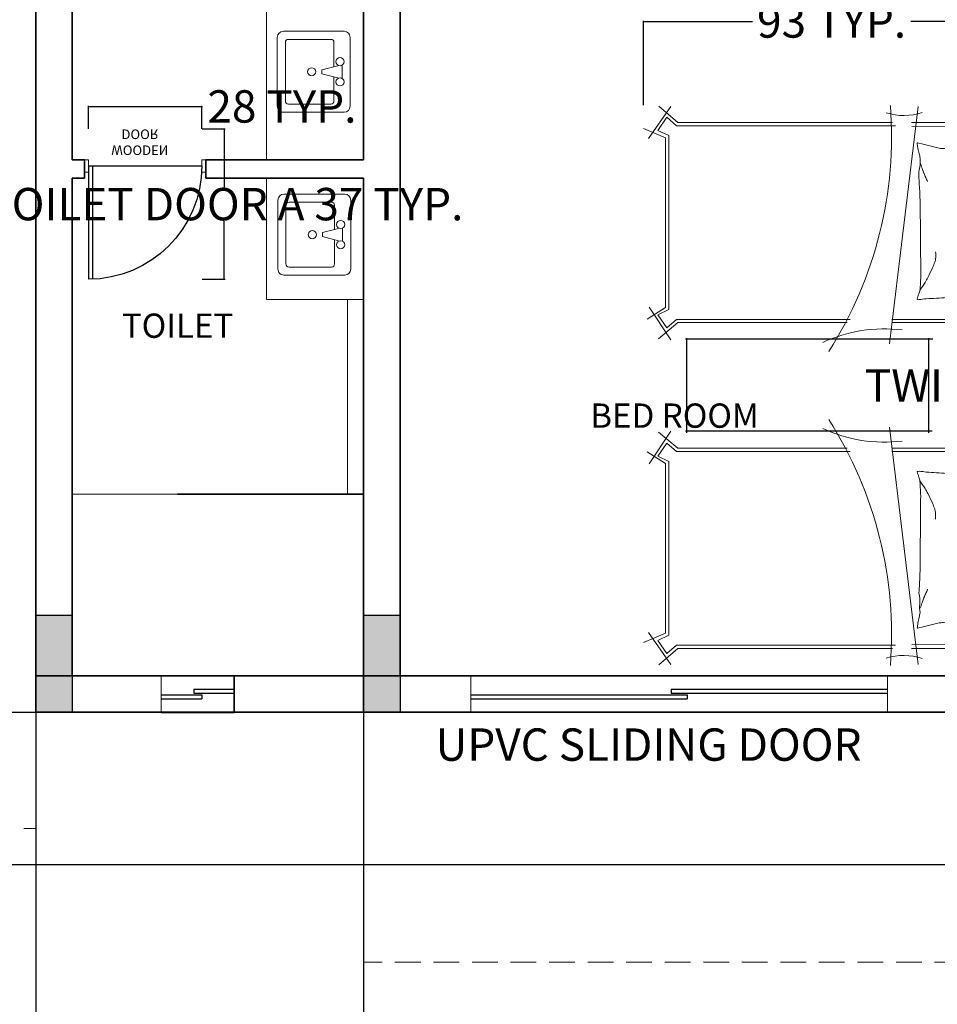
# Model space of a CAD drawing. Units: inches. Extents: x -48 to 50072, y 0 to 21068.
# Tile 51 of 75: x 212 to 439, y 417 to 660. Entities that reach past the tile are written whole.
import ezdxf

# ---------------------------------------------------------------- set-up
doc = ezdxf.new("R2010")
doc.units = ezdxf.units.IN
doc.header["$MEASUREMENT"] = 0
doc.linetypes.add('HIDDEN', pattern=[9.525, 6.35, -3.175])
for name, color, linetype, lineweight in [('A-ANNO-DIMS', 2, 'Continuous', 18), ('A-ANNO-TEXT', 7, 'Continuous', 18), ('A-AREA-IDEN', 7, 'Continuous', 18), ('A-COLS', 1, 'Continuous', 35), ('A-DOOR', 4, 'Continuous', 18), ('A-FLOR-CASE', 9, 'Continuous', 18), ('A-FLOR-FIXT', 4, 'Continuous', 18), ('A-FLOR-OVHD', 8, 'HIDDEN', 13), ('A-GLAZ', 4, 'Continuous', 18), ('A-WALL', 7, 'Continuous', 35), ('FURNITURE', 44, 'Continuous', 18)]:
    doc.layers.add(name, color=color, linetype=linetype, lineweight=lineweight)
for name, color, linetype in [('Layer3', 176, 'Continuous'), ('家具1', 1, 'Continuous'), ('家具１', 1, 'Continuous')]:
    doc.layers.add(name, color=color, linetype=linetype)
doc.styles.get("Standard").update_dxf_attribs({"font": 'arial.ttf'})
doc.dimstyles.get("Standard").update_dxf_attribs({"dimtxt": 8, "dimasz": 0.18, "dimexe": 0.18, "dimexo": 0.0625, "dimgap": 0.09, "dimtad": 0, "dimtih": 1, "dimtoh": 1, "dimdec": 1, "dimzin": 0, "dimdsep": 46, "dimlunit": 4, "dimtxsty": 'Standard', "dimblk": 'ARCHTICK', "dimcen": 0.09, "dimadec": 0, "dimazin": 0, "dimtfac": 1, "dimtdec": 1, "dimtofl": 0, "dimtmove": 0, "dimatfit": 3, "dimldrblk": 'ARCHTICK', "dimfxl": 1, "dimtolj": 1, "dimtzin": 0, "dimarcsym": 0})

# ---------------------------------------------------------------- blocks, each defined once
blk = doc.blocks.new('bnniku')
at = {"layer": 'Defpoints'}
h = blk.add_hatch(color=256, dxfattribs=at)
h.dxf.hatch_style = 1
h.paths.add_polyline_path([(767.55, 1114.04), (758.55, 1114.04), (758.55, 1090.04), (767.55, 1090.04)])
for p, q in [((758.55, 1114.04), (767.55, 1114.04)), ((758.55, 1090.04), (758.55, 1114.04)), ((767.55, 1114.04), (767.55, 1090.04)), ((767.55, 1090.04), (758.55, 1090.04))]:
    blk.add_line(p, q, dxfattribs=at)
blk = doc.blocks.new('gthyerhy')
at = {"layer": 'Defpoints'}
for p, q in [((665.59, 603.33), (665.59, 631.33)), ((666.59, 603.33), (666.59, 631.32)), ((665.59, 603.33), (693.59, 603.33))]:
    blk.add_line(p, q, dxfattribs=at)
blk.add_arc((665.59, 603.33), 28, 0, 90, dxfattribs=at)
at = {"insert": (674.82, 600.63), "char_height": 2.3647, "attachment_point": 1}
blk.add_mtext_dynamic_manual_height_columns('\\pxqc;WOODEN ^JDOOR', width=6.8949, gutter_width=11.82, heights=[0], dxfattribs=at)
blk = doc.blocks.new('jyugcli')
for p, q in [((342.02, 1025.77), (342.02, 1034.77)), ((360.02, 1025.77), (360.02, 1034.77))]:
    blk.add_line(p, q)
at = {"layer": 'Defpoints'}
for p, q in [((342.02, 1030.07), (352.02, 1030.07)), ((350.02, 1031.47), (360.02, 1031.47)), ((350.02, 1031.47), (350.02, 1030.47)), ((350.02, 1030.47), (360.02, 1030.47)), ((352.02, 1030.07), (352.02, 1029.07)), ((342.02, 1029.07), (352.02, 1029.07))]:
    blk.add_line(p, q, dxfattribs=at)
at = {"layer": 'Layer3'}
for p, q in [((342.02, 1034.77), (360.02, 1034.77)), ((342.02, 1025.77), (360.02, 1025.77))]:
    blk.add_line(p, q, dxfattribs=at)
blk = doc.blocks.new('fdsghhhhhhygr')
for p, q in [((41.77, 686.77), (41.77, 677.77)), ((144.77, 677.77), (144.77, 686.77))]:
    blk.add_line(p, q)
at = {"layer": 'Defpoints'}
for p, q in [((41.77, 682.07), (95.27, 682.07)), ((91.27, 683.47), (144.77, 683.47)), ((91.27, 683.47), (91.27, 682.47)), ((91.27, 682.47), (144.77, 682.47)), ((95.27, 682.07), (95.27, 681.07)), ((41.77, 681.07), (95.27, 681.07))]:
    blk.add_line(p, q, dxfattribs=at)
at = {"layer": 'Layer3'}
for p, q in [((41.77, 686.77), (144.77, 686.77)), ((144.77, 677.77), (41.77, 677.77))]:
    blk.add_line(p, q, dxfattribs=at)
blk = doc.blocks.new('A$C7A8469D8')
for p, q in [((105.4, 2275.5), (1345.4, 2275.5)), ((105.4, 1660.8), (105.4, 2275.5)), ((1345.4, 2275.5), (1345.4, 1540.4)), ((3363.9, 2275.5), (2123.9, 2275.5)), ((2123.9, 2275.5), (2123.9, 1540.4)), ((3363.9, 1660.8), (3363.9, 2275.5)), ((1345.4, 2255.5), (105.4, 2255.5)), ((1325.4, 2205.5), (125.4, 2205.5)), ((129.2, 1662.5), (125.4, 2205.5)), ((1325.4, 1539.2), (1325.4, 2205.5)), ((2123.9, 2255.5), (3363.9, 2255.5)), ((2143.9, 2205.5), (3343.9, 2205.5)), ((2143.9, 1539.2), (2143.9, 2205.5)), ((3340.1, 1662.5), (3343.9, 2205.5)), ((963.7, 2086.6), (963.7, 2086.6)), ((963.7, 2086.6), (963.7, 2086.6)), ((997.2, 2115.8), (997.2, 2115.8)), ((2472.1, 2115.8), (2472.1, 2115.8)), ((2505.6, 2086.6), (2505.6, 2086.6)), ((2505.6, 2086.6), (2505.6, 2086.6)), ((284, 2013), (284, 2013)), ((284, 2013), (284, 2013)), ((940.8, 2061.8), (940.8, 2061.8)), ((2528.5, 2061.8), (2528.5, 2061.8)), ((3185.3, 2013), (3185.3, 2013)), ((3185.3, 2013), (3185.3, 2013)), ((239.9, 1733), (264.7, 1832.1)), ((3229.5, 1733), (3204.7, 1832.1)), ((230.9, 1697), (239.9, 1733)), ((1064.8, 1762.3), (1064.8, 1762.3)), ((1096.9, 1744.2), (1096.9, 1744.2)), ((1096.9, 1744.2), (1096.9, 1744.2)), ((1096.9, 1744.2), (1096.9, 1744.2)), ((2372.4, 1744.2), (2372.4, 1744.2)), ((2372.4, 1744.2), (2372.4, 1744.2)), ((2372.4, 1744.2), (2372.4, 1744.2)), ((2404.5, 1762.3), (2404.5, 1762.3)), ((3238.5, 1697), (3229.5, 1733)), ((1476.1, 1524.8), (6.4, 1700.6)), ((230.9, 1697), (230.5, 1695.5)), ((1993.2, 1524.8), (3462.9, 1700.6)), ((3238.5, 1697), (3238.8, 1695.5)), ((105.4, 212.1), (105.4, 1542.9)), ((125.4, 204.7), (125.4, 1561.6)), ((3343.9, 204.7), (3343.9, 1561.6)), ((3363.9, 212.1), (3363.9, 1542.9)), ((1325.4, 204.7), (1325.4, 1280.1)), ((1345.4, 1261.4), (1345.4, 212.1)), ((2123.9, 1261.4), (2123.9, 212.1)), ((2143.9, 204.7), (2143.9, 1280.1)), ((4.4, 94.3), (105.4, 212.1)), ((125.4, 204.7), (73.3, 144)), ((1325.4, 204.7), (1377.6, 144)), ((1345.4, 212.1), (1446.2, 92.2)), ((2123.9, 212.1), (2023.1, 92.2)), ((2143.9, 204.7), (2091.7, 144)), ((3343.9, 204.7), (3396, 144)), ((3464.9, 94.3), (3363.9, 212.1)), ((203.9, 30), (6.6, 169.4)), ((73.3, 144), (154.5, 88.5)), ((199.5, 135.5), (141.7, 0)), ((154.5, 88.5), (186.9, 155.5)), ((186.9, 155.5), (1264, 155.5)), ((1251.4, 135.5), (199.5, 135.5)), ((1452.6, 169.4), (1248.8, 34.3)), ((1323.9, 21.4), (1251.4, 135.5)), ((1296.4, 88.5), (1264, 155.5)), ((1377.6, 144), (1296.4, 88.5)), ((2016.7, 169.4), (2220.5, 34.3)), ((2091.7, 144), (2172.9, 88.5)), ((2145.4, 21.4), (2217.9, 135.5)), ((2172.9, 88.5), (2205.3, 155.5)), ((3282.4, 155.5), (2205.3, 155.5)), ((2217.9, 135.5), (3269.8, 135.5)), ((3265.4, 30), (3462.8, 169.4)), ((3269.8, 135.5), (3327.6, 0)), ((3314.8, 88.5), (3282.4, 155.5)), ((3396, 144), (3314.8, 88.5))]:
    blk.add_line(p, q)
for centre, radius, start, end in [((227.2, 2136.4), 15.7, 101.27238, 206.58052), ((245.3, 2045.5), 108.5, 90, 101.27238), ((245.3, 1960.6), 193.4, 81.56281, 90), ((220, 1790.1), 365.7, 74.25602, 81.56281), ((398.1, 2421.9), 290.7, 254.25602, 262.45315), ((201.4, 24611.4), 22481.3, 271.01841, 271.70805), ((903.9, 1960.2), 182.9, 92.53859, 100.18988), ((911.2, 1795.5), 347.6, 85.19815, 92.53859), ((1028, 3186.1), 1047.8, 265.19815, 269.42426), ((1140.8, 1875.8), 280.8, 110.86028, 117.23959), ((1035.5, 3931.4), 1793.1, 269.42426, 271.90789), ((1130.4, 2026.4), 119, 105.93524, 126.08636), ((1062.4, 3123.6), 984.9, 271.90789, 275.25919), ((1130.4, 2026.4), 119, 85.78412, 105.93524), ((1146.7, 2207.3), 64.7, 275.25919, 300.65125), ((1197.4, 2121.8), 34.7, 85.69746, 120.65125), ((1197.7, 2126.3), 30.1, 68.2117, 85.69746), ((1219.6, 2138.1), 18.7, 158.0096, 201.42098), ((1207, 2143.2), 5.13, 78.10694, 158.0096), ((1208.6, 2150.9), 2.78, 258.10694, 19.56397), ((1207.4, 2150.5), 4.1, 19.56397, 68.2117), ((2256.5, 2155.7), 4.1, 291.7883, 340.43603), ((2258.6, 2149.1), 2.78, 340.43603, 101.89306), ((2258.1, 2184.3), 30.1, 274.30254, 291.7883), ((2266, 2150.1), 5.13, 201.9904, 281.89306), ((2284.5, 2138.3), 18.7, 158.57902, 201.9904), ((2287, 2186.2), 34.7, 239.34875, 274.30254), ((2283.7, 2087.2), 64.7, 59.34875, 84.74081), ((2283.9, 1158.4), 984.9, 84.74081, 88.09211), ((2362.9, 2259.6), 119, 254.06476, 274.21588), ((2441.7, 2237), 119, 233.91364, 254.06476), ((2392.2, 346.2), 1793.1, 88.09211, 90.57574), ((2557.1, 2387.9), 280.8, 242.76041, 249.13972), ((2539.6, 1094.2), 1047.8, 90.57574, 94.80185), ((2544.4, 2489.3), 347.6, 267.46141, 274.80185), ((2605.9, 2322.8), 182.9, 259.81012, 267.46141), ((2198.2, -20337.6), 22481.3, 88.29195, 88.98159), ((3188.3, 1853.9), 290.7, 97.54685, 105.74398), ((3096.4, 2503.8), 365.7, 278.43719, 285.74398), ((3195.6, 2345.2), 193.4, 270, 278.43719), ((3245.2, 2260.3), 108.5, 258.72762, 270), ((3259.3, 2144.8), 15.7, 153.41948, 258.72762), ((249.8, 2147.7), 41, 206.58052, 265.59979), ((833.2, 2043.1), 590.2, 173.76764, 180), ((180.9, 2000.6), 107.8, 41.44291, 53.73593), ((169.6, 1957.5), 167.9, 45.09762, 62.79641), ((169.6, 1957.5), 167.9, 27.39883, 45.09762), ((467.5, 2945.8), 819.2, 262.45315, 270), ((467.5, 3385.4), 1258.8, 270, 276.0867), ((1150.7, 1891.6), 270.2, 133.81151, 140.96506), ((1150.7, 1891.6), 270.2, 133.8115, 140.96506), ((1150.7, 1891.6), 270.2, 133.8115, 140.96506), ((1289, 1747.4), 470, 128.38857, 133.81151), ((1289, 1747.4), 470, 128.38857, 133.81151), ((1289, 1747.4), 470, 128.38857, 133.8115), ((1054.4, 2043.6), 92.1, 117.23959, 128.38857), ((1130.4, 2026.4), 119, 143.82335, 161.56035), ((1130.4, 2026.4), 119, 126.08636, 143.82335), ((1433.6, 2041.2), 238, 167.89054, 172.3191), ((912.2, 2153.1), 295.2, 347.89054, 351.86652), ((1165.5, 2116.9), 39.3, 351.86652, 21.42098), ((2228.2, 2125.7), 39.3, 338.57902, 8.13348), ((1976.2, 2049.4), 295.2, 8.13348, 12.10946), ((2504.3, 2123), 238, 187.6809, 192.10946), ((2505.1, 2192.8), 119, 216.17665, 233.91364), ((2548, 2134.3), 119, 198.43965, 216.17665), ((2514.3, 2197.7), 92.1, 231.61143, 242.76041), ((2797.5, 2455), 470, 226.18849, 231.61143), ((2180.3, 1747.4), 470, 46.18849, 51.61143), ((2180.3, 1747.4), 470, 46.1885, 51.61143), ((2715.6, 2256.8), 270.2, 219.03494, 226.18849), ((2318.6, 1891.6), 270.2, 39.03494, 46.1885), ((2318.6, 1891.6), 270.2, 39.03494, 46.1885), ((2868.3, 874.9), 1258.8, 83.9133, 90), ((3109.4, 1314.5), 819.2, 90, 97.54685), ((3032, 2153.7), 167.9, 314.90238, 332.60117), ((3104.4, 2225.8), 167.9, 297.20359, 314.90238), ((3143.8, 2159), 107.8, 306.26407, 318.55709), ((3259.4, 2088.4), 41, 94.40021, 153.41948), ((3813.1, 2107.2), 590.2, 180, 186.23236), ((487.7, 2043.1), 244.8, 180, 189.68437), ((214.4, 2030.2), 63.1, 25.35512, 41.44291), ((107.6, 1979.6), 181.3, 21.81492, 25.35512), ((46.9, 1955.3), 246.7, 18.7799, 21.81492), ((216.6, 2013), 67.4, 0, 18.7799), ((174.2, 2013), 109.8, 345.31489, 360), ((169.6, 1957.5), 167.9, 16.51498, 27.39883), ((1146.2, 1938.6), 240.2, 151.68324, 156.99723), ((986.8, 2024.5), 59.2, 140.96506, 151.68324), ((2283.6, 1926.6), 1095.7, 172.3191, 176.63125), ((3365.4, 2137.4), 1095.7, 183.36875, 187.6809), ((2580.6, 2089.8), 59.2, 208.31676, 219.03494), ((2755.7, 2146.4), 240.2, 203.00277, 208.31676), ((2989.6, 2082.5), 167.9, 332.60117, 343.48502), ((3121.5, 2034.7), 67.4, 341.2201, 360), ((3079.1, 1985.2), 109.8, 0, 14.68511), ((2959.9, 2126.4), 246.7, 338.18508, 341.2201), ((3029.6, 2124.6), 181.3, 334.64488, 338.18508), ((3150.6, 2099), 63.1, 318.55709, 334.64488), ((3467.6, 2001.9), 244.8, 170.31563, 180), ((1289.8, 2180), 1058.4, 189.68437, 192.19838), ((-116.7, 1875.9), 380.5, 8.00505, 12.19838), ((169.6, 1957.5), 167.9, 5.63113, 16.51498), ((2002.9, 1943.1), 814.5, 176.63125, 181.63309), ((3093.7, 1967.8), 814.5, 178.36691, 183.36875), ((2971.5, 2021.7), 167.9, 343.48502, 354.36887), ((2837.2, 2009.3), 380.5, 347.80162, 351.99495), ((4257.4, 1778.3), 1058.4, 167.80162, 170.31563), ((-522.7, 1818.8), 790.5, 2.66488, 8.00505), ((2826.3, 1966.6), 1638.3, 181.63309, 183.05496), ((3916.5, 1832.6), 1638.3, 176.94504, 178.36691), ((2419.5, 1965.7), 790.5, 351.99495, 357.33512), ((185.8, 1851.8), 81.3, 345.95481, 2.66488), ((17529.8, 2751.3), 16362.7, 183.05496, 183.50486), ((18611, 879), 16362.7, 176.49514, 176.94504), ((3123.5, 1835.8), 81.3, 357.33512, 14.04519), ((927.3, 1483.7), 326.5, 85.91723, 93.5552), ((945.6, 1740), 69.6, 69.32572, 85.91723), ((755.5, 1236.2), 608, 65.67347, 69.32572), ((297.9, 224.1), 1718.7, 63.50152, 65.67347), ((1696.5, 3328.4), 1718.7, 294.32653, 296.49848), ((2248.7, 2359), 608, 290.67428, 294.32653), ((2494.2, 1874.4), 69.6, 274.08277, 290.67428), ((2539, 2135.2), 326.5, 266.4448, 274.08277), ((-288.1, 1611.6), 350.3, 341.98878, 19.11363), ((217, 1971), 275.6, 279.4841, 287.38641), ((342.3, 1570.9), 143.7, 96.43405, 107.38641), ((345.8, 1539.7), 175.1, 78.44144, 96.43405), ((93, 2561.3), 886.4, 287.19822, 289.42798), ((436.2, 1981.7), 276.1, 258.44144, 272.74906), ((93, 2561.3), 886.4, 289.42674, 291.8864), ((93, 2561.3), 886.4, 289.42798, 291.65774), ((93, 2561.3), 886.4, 289.42831, 291.55903), ((93, 2561.3), 886.4, 289.42674, 289.42831), ((93, 2561.3), 886.4, 291.42998, 291.72586), ((93, 2561.3), 886.4, 291.42998, 291.71), ((93, 2561.3), 886.4, 291.44301, 291.83448), ((93, 2561.3), 886.4, 291.44301, 291.48398), ((93, 2561.3), 886.4, 291.48398, 291.72586), ((93, 2561.3), 886.4, 291.55903, 291.83448), ((93, 2561.3), 886.4, 291.65774, 293.48441), ((93, 2561.3), 886.4, 291.71, 291.8864), ((93, 2561.3), 886.4, 293.48441, 295.31107), ((368.6, 3389.7), 1685.7, 272.74906, 274.61758), ((621.8, 254.5), 1459.7, 92.60963, 94.61758), ((1098, -33470.9), 35187.8, 90.32849, 90.88356), ((1012.4, -5144.9), 6862.2, 89.71346, 90.97038), ((1039.8, 320.4), 1396.8, 86.42603, 89.71346), ((897.4, 1426.5), 375.2, 57.86502, 63.50152), ((897.4, 1426.5), 375.2, 57.86501, 63.50152), ((897.4, 1426.5), 375.2, 57.86502, 63.50152), ((631.9, 1003.8), 874.3, 54.17371, 57.86502), ((1115.9, 1539.8), 175.1, 77.13096, 86.42603), ((1142.8, 1657.5), 54.3, 62.71588, 77.13096), ((1582.4, 1774.6), 385.4, 183.50486, 189.99836), ((2651.1, 1684.1), 385.4, 170.00164, 176.49514), ((2289.5, 1758.8), 54.3, 282.86904, 297.28412), ((2303.5, 1885.2), 175.1, 273.57397, 282.86904), ((1860.6, 2453.1), 874.3, 302.13498, 305.82629), ((2335.5, 3111.3), 1396.8, 270.28654, 273.57397), ((2205, 2080), 375.2, 296.49848, 302.13498), ((2571.9, 1426.5), 375.2, 116.49848, 122.13499), ((2571.9, 1426.5), 375.2, 116.49848, 122.13498), ((2538.8, 8578.4), 6862.2, 269.02962, 270.28654), ((3115.7, 36899.9), 35187.8, 269.11644, 269.67151), ((3031.5, 3167.7), 1459.7, 265.38242, 267.39037), ((2884.2, 25.7), 1685.7, 85.38242, 87.25094), ((2644.1, 947), 886.4, 64.68893, 66.51559), ((3075.2, 1435.5), 276.1, 87.25094, 101.55856), ((2695.9, 924.5), 886.4, 66.51559, 68.34226), ((3376.3, 2561.3), 886.4, 248.1136, 250.57326), ((3376.3, 2561.3), 886.4, 248.1136, 248.29), ((3376.3, 2561.3), 886.4, 248.16552, 248.55699), ((3376.3, 2561.3), 886.4, 248.16552, 248.44097), ((3376.3, 2561.3), 886.4, 248.27414, 248.57002), ((3376.3, 2561.3), 886.4, 248.27414, 248.51602), ((3376.3, 2561.3), 886.4, 248.29, 248.57002), ((2754.3, 901.6), 886.4, 68.34226, 70.57202), ((3376.3, 2561.3), 886.4, 248.44097, 250.57169), ((3376.3, 2561.3), 886.4, 248.51602, 248.55699), ((3376.3, 2561.3), 886.4, 250.57169, 250.57326), ((2819.4, 878.6), 886.4, 70.57202, 72.80178), ((3108.1, 1885.2), 175.1, 263.56595, 281.55856), ((3186.1, 1850.8), 143.7, 252.61359, 263.56595), ((3124.6, 1436.2), 275.6, 72.61359, 80.5159), ((3757.4, 1611.6), 350.3, 160.88637, 198.01122), ((208.9, 2019.7), 324.9, 273.81546, 274.08294), ((231.9, 1696.7), 1.1, 165.95461, 274.08286), ((231.9, 1696.7), 1.1, 165.95506, 274.08294), ((208.9, 2019.7), 324.9, 274.08294, 279.4841), ((1209.9, 1787.6), 92.1, 242.71588, 253.77885), ((1213.5, 1800), 105, 253.77885, 262.87961), ((1200.7, 1697.4), 1.59, 262.87961, 343.30223), ((1180, 1703.6), 23.2, 343.30223, 9.99836), ((2244.2, 1701), 23.2, 350.00164, 16.69777), ((2267.3, 1695.4), 1.59, 16.69777, 97.12039), ((2298.1, 1595), 105, 97.12039, 106.22115), ((2327.3, 1617.4), 92.1, 106.22115, 117.28412), ((3183.8, 1375.1), 324.9, 80.5159, 85.91706), ((3237.4, 1696.7), 1.1, 265.91714, 14.04539), ((3238.4, 1695.9), 1.1, 85.91706, 194.04494), ((3260.5, 2019.7), 324.9, 265.91706, 266.18454), ((2296.9, 1493), 913.1, 173.14417, 204.73358), ((1172.5, 1493), 913.1, 335.26642, 6.85583), ((191.6, -937), 2473.5, 57.42475, 94.44158), ((3277.8, -937), 2473.5, 85.55842, 122.57525)]:
    blk.add_arc(centre, radius, start, end)
at = {"layer": '家具1'}
for p, q in [((1613.7, 2082.3), (1613.7, 2329.8)), ((1836.1, 2082.3), (1836.1, 2329.8)), ((100.7, 2292.6), (0.7, 2292.6)), ((0.7, 2292.6), (0.7, 2192.6)), ((100.7, 2292.6), (100.7, 2192.6)), ((1348.1, 2292.6), (1448.1, 2292.6)), ((1348.1, 2292.6), (1348.1, 2192.6)), ((2031.9, 2292.6), (1440.5, 2292.6)), ((1448.1, 2303.2), (1448.1, 1885)), ((1448.1, 2292.6), (1448.1, 2192.6)), ((2018.1, 2303.2), (2018.1, 1885)), ((2121.2, 2292.6), (2021.2, 2292.6)), ((2021.2, 2292.6), (2021.2, 2192.6)), ((2121.2, 2292.6), (2121.2, 2192.6)), ((3368.6, 2292.6), (3468.6, 2292.6)), ((3368.6, 2292.6), (3368.6, 2192.6)), ((1518.4, 2196.5), (1709, 2196.5)), ((1757, 2205.5), (1695.7, 2205.5)), ((1740.8, 2196.5), (1931.4, 2196.5)), ((100.7, 2192.6), (0.7, 2192.6)), ((1348.1, 2192.6), (1448.1, 2192.6)), ((1757, 2185.5), (1695.7, 2185.5)), ((2121.2, 2192.6), (2021.2, 2192.6)), ((3368.6, 2192.6), (3468.6, 2192.6)), ((2028.8, 1892.6), (1440.5, 1892.6)), ((1448.1, 1792.9), (1448.1, 260.3)), ((2018.1, 1787.6), (2018.1, 260.3)), ((2028.8, 1767.9), (1440.5, 1767.9)), ((2028.8, 267.9), (1440.5, 267.9))]:
    blk.add_line(p, q, dxfattribs=at)
for centre, radius in [((50.7, 2242.6), 40), ((1398.1, 2242.6), 40), ((1616.3, 2195.5), 80), ((1836.3, 2195.5), 80), ((2071.2, 2242.6), 40), ((3418.6, 2242.6), 40)]:
    blk.add_circle(centre, radius, dxfattribs=at)
at = {"layer": '家具１'}
blk.add_line((3468.6, 2292.6), (3468.6, 2192.6), dxfattribs=at)
blk = doc.blocks.new('A$C329C6BD7')
at = {"linetype": 'ByBlock'}
for p, q in [((0.4699, 0.4572), (0.0381, 0.4572)), ((0, 0.4191), (0, 0.0381)), ((0.2159, 0.4064), (0.2921, 0.4064)), ((0.2159, 0.381), (0.2413, 0.2794)), ((0.2667, 0.2794), (0.2921, 0.381)), ((0.508, 0.0381), (0.508, 0.4191)), ((0.0508, 0.0698), (0.0508, 0.3365)), ((0.0698, 0.3556), (0.2223, 0.3556)), ((0.2858, 0.3556), (0.4382, 0.3556)), ((0.4572, 0.3365), (0.4572, 0.0698)), ((0.2413, 0.2794), (0.2667, 0.2794)), ((0.4382, 0.0508), (0.0698, 0.0508)), ((0.0381, 0), (0.4699, 0))]:
    blk.add_line(p, q, dxfattribs=at)
for centre in [(0.1905, 0.3937), (0.3175, 0.3937), (0.254, 0.2159)]:
    blk.add_circle(centre, 0.0254, dxfattribs=at)
for centre, radius, start, end in [((0.0381, 0.4191), 0.0381, 90, 180), ((0.4699, 0.4191), 0.0381, 0, 90), ((0.0698, 0.3365), 0.0191, 90, 180), ((0.4382, 0.3365), 0.0191, 0, 90), ((0.0698, 0.0698), 0.0191, 180, 270), ((0.4382, 0.0698), 0.0191, 270, 0), ((0.0381, 0.0381), 0.0381, 180, 270), ((0.4699, 0.0381), 0.0381, 270, 0)]:
    blk.add_arc(centre, radius, start, end, dxfattribs=at)
blk = doc.blocks.new('DOOR-ENTRY-TANDEM-48')
for p, q in [((2, 43), (2, 86)), ((3, 85.99), (3, 43)), ((0, 45), (2, 45)), ((2, 41), (2, 45)), ((46, 41), (46, 45)), ((46, 45), (48, 45)), ((2, 43), (3, 43)), ((2, 43), (3, 43)), ((2, 43), (3, 43)), ((45, 0), (45, 43)), ((45, 43), (46, 43)), ((46, 43), (46, 7)), ((0, 41), (48, 41)), ((46, 7), (46, 0.01))]:
    blk.add_line(p, q)
for centre, start, end in [((2, 43), 0, 90), ((45, 43), 180, 271.3326)]:
    blk.add_arc(centre, 43, start, end)
blk = doc.blocks.new('_ArchTick')
at = {"color": 0, "linetype": 'ByBlock', "const_width": 0.15}
blk.add_lwpolyline([(-0.5, -0.5), (0.5, 0.5)], dxfattribs=at)
blk = doc.blocks.new('*D68')
at = {"layer": 'A-ANNO-DIMS', "color": 0, "lineweight": -2, "transparency": 16777216}
for p, q in [((257.08, 632.91), (262.77, 632.91)), ((262.59, 632.91), (262.59, 618.57)), ((262.59, 595.77), (262.59, 610.11)), ((257.08, 595.77), (262.77, 595.77))]:
    blk.add_line(p, q, dxfattribs=at)
at = {"layer": 'Defpoints', "color": 0, "transparency": 16777216}
for p in [(257.02, 632.91), (257.02, 595.77), (262.59, 595.77)]:
    blk.add_point(p, dxfattribs=at)
at = {"layer": 'A-ANNO-DIMS', "color": 0, "lineweight": -2, "transparency": 16777216, "xscale": 0.18, "yscale": 0.18, "zscale": 0.18}
for p, rotation in [((262.59, 632.91), 90), ((262.59, 595.77), 270)]:
    blk.add_blockref('_ArchTick', p, dxfattribs=dict(at, rotation=rotation))
at = {"layer": 'A-ANNO-DIMS', "color": 0, "transparency": 16777216, "insert": (262.59, 614.34), "char_height": 8, "attachment_point": 5}
blk.add_mtext('\\A1;TOILET DOOR A 37 TYP.', dxfattribs=at)
blk = doc.blocks.new('*D69')
at = {"layer": 'A-ANNO-DIMS', "color": 0, "lineweight": -2, "transparency": 16777216}
for p, q in [((229.02, 632.97), (229.02, 638.66)), ((229.02, 638.48), (257.02, 638.48)), ((257.02, 632.97), (257.02, 638.66)), ((257.02, 638.48), (257.2, 638.48))]:
    blk.add_line(p, q, dxfattribs=at)
at = {"layer": 'Defpoints', "color": 0, "transparency": 16777216}
for p in [(257.02, 638.48), (229.02, 632.91), (257.02, 632.91)]:
    blk.add_point(p, dxfattribs=at)
at = {"layer": 'A-ANNO-DIMS', "color": 0, "lineweight": -2, "transparency": 16777216, "xscale": 0.18, "yscale": 0.18, "zscale": 0.18, "rotation": 180}
blk.add_blockref('_ArchTick', (229.02, 638.48), dxfattribs=at)
at = {"layer": 'A-ANNO-DIMS', "color": 0, "lineweight": -2, "transparency": 16777216, "xscale": 0.18, "yscale": 0.18, "zscale": 0.18}
blk.add_blockref('_ArchTick', (257.02, 638.48), dxfattribs=at)
at = {"layer": 'A-ANNO-DIMS', "color": 0, "transparency": 16777216, "insert": (276.83, 638.48), "char_height": 8, "attachment_point": 5}
blk.add_mtext('\\A1;28 TYP.', dxfattribs=at)
blk = doc.blocks.new('*D74')
at = {"layer": 'A-ANNO-DIMS', "color": 0, "lineweight": -2, "transparency": 16777216}
for p, q in [((459.18, 638.72), (480.05, 638.72)), ((479.87, 638.72), (479.87, 573.76)), ((479.87, 500.35), (479.87, 565.3)), ((459.18, 500.35), (480.05, 500.35))]:
    blk.add_line(p, q, dxfattribs=at)
at = {"layer": 'Defpoints', "color": 0, "transparency": 16777216}
for p in [(459.12, 638.72), (459.12, 500.35), (479.87, 500.35)]:
    blk.add_point(p, dxfattribs=at)
at = {"layer": 'A-ANNO-DIMS', "color": 0, "lineweight": -2, "transparency": 16777216, "xscale": 0.18, "yscale": 0.18, "zscale": 0.18}
for p, rotation in [((479.87, 638.72), 90), ((479.87, 500.35), 270)]:
    blk.add_blockref('_ArchTick', p, dxfattribs=dict(at, rotation=rotation))
at = {"layer": 'A-ANNO-DIMS', "color": 0, "transparency": 16777216, "insert": (479.87, 569.53), "char_height": 8, "attachment_point": 5}
blk.add_mtext('\\A1;TWIN BED SET 138 TYP.', dxfattribs=at)
blk = doc.blocks.new('*D75')
at = {"layer": 'A-ANNO-DIMS', "color": 0, "lineweight": -2, "transparency": 16777216}
for p, q in [((366.2, 638.78), (366.2, 659.65)), ((366.2, 659.47), (393.1, 659.47)), ((459.12, 659.47), (432.22, 659.47)), ((459.12, 638.78), (459.12, 659.65))]:
    blk.add_line(p, q, dxfattribs=at)
at = {"layer": 'Defpoints', "color": 0, "transparency": 16777216}
for p in [(459.12, 659.47), (366.2, 638.72), (459.12, 638.72)]:
    blk.add_point(p, dxfattribs=at)
at = {"layer": 'A-ANNO-DIMS', "color": 0, "lineweight": -2, "transparency": 16777216, "xscale": 0.18, "yscale": 0.18, "zscale": 0.18, "rotation": 180}
blk.add_blockref('_ArchTick', (366.2, 659.47), dxfattribs=at)
at = {"layer": 'A-ANNO-DIMS', "color": 0, "lineweight": -2, "transparency": 16777216, "xscale": 0.18, "yscale": 0.18, "zscale": 0.18}
blk.add_blockref('_ArchTick', (459.12, 659.47), dxfattribs=at)
at = {"layer": 'A-ANNO-DIMS', "color": 0, "transparency": 16777216, "insert": (412.66, 659.47), "char_height": 8, "attachment_point": 5}
blk.add_mtext('\\A1;93 TYP.', dxfattribs=at)
blk = doc.blocks.new('*D116')
at = {"layer": 'A-ANNO-DIMS', "color": 0, "lineweight": -2, "transparency": 16777216}
for p, q in [((18.02, 677.71), (18.02, 165.94)), ((216.02, 677.71), (216.02, 165.94)), ((18.02, 166.12), (108.46, 166.12)), ((216.02, 166.12), (125.58, 166.12))]:
    blk.add_line(p, q, dxfattribs=at)
at = {"layer": 'Defpoints', "color": 0, "transparency": 16777216}
for p in [(18.02, 677.77), (216.02, 677.77), (216.02, 166.12)]:
    blk.add_point(p, dxfattribs=at)
at = {"layer": 'A-ANNO-DIMS', "color": 0, "lineweight": -2, "transparency": 16777216, "xscale": 0.18, "yscale": 0.18, "zscale": 0.18, "rotation": 180}
blk.add_blockref('_ArchTick', (18.02, 166.12), dxfattribs=at)
at = {"layer": 'A-ANNO-DIMS', "color": 0, "lineweight": -2, "transparency": 16777216, "xscale": 0.18, "yscale": 0.18, "zscale": 0.18}
blk.add_blockref('_ArchTick', (216.02, 166.12), dxfattribs=at)
at = {"layer": 'A-ANNO-DIMS', "color": 0, "transparency": 16777216, "insert": (117.02, 166.12), "char_height": 8, "attachment_point": 5}
blk.add_mtext('\\A1;198', dxfattribs=at)
blk = doc.blocks.new('*D117')
at = {"layer": 'A-ANNO-DIMS', "color": 0, "lineweight": -2, "transparency": 16777216}
for p, q in [((216.02, 488.71), (216.02, 165.94)), ((297.02, 488.71), (297.02, 165.94)), ((216.02, 166.12), (251.46, 166.12)), ((297.02, 166.12), (261.57, 166.12))]:
    blk.add_line(p, q, dxfattribs=at)
at = {"layer": 'Defpoints', "color": 0, "transparency": 16777216}
for p in [(216.02, 488.77), (297.02, 488.77), (297.02, 166.12)]:
    blk.add_point(p, dxfattribs=at)
at = {"layer": 'A-ANNO-DIMS', "color": 0, "lineweight": -2, "transparency": 16777216, "xscale": 0.18, "yscale": 0.18, "zscale": 0.18, "rotation": 180}
blk.add_blockref('_ArchTick', (216.02, 166.12), dxfattribs=at)
at = {"layer": 'A-ANNO-DIMS', "color": 0, "lineweight": -2, "transparency": 16777216, "xscale": 0.18, "yscale": 0.18, "zscale": 0.18}
blk.add_blockref('_ArchTick', (297.02, 166.12), dxfattribs=at)
at = {"layer": 'A-ANNO-DIMS', "color": 0, "transparency": 16777216, "insert": (256.52, 166.12), "char_height": 8, "attachment_point": 5}
blk.add_mtext('\\A1;81', dxfattribs=at)
blk = doc.blocks.new('*D118')
at = {"layer": 'A-ANNO-DIMS', "color": 0, "lineweight": -2, "transparency": 16777216}
for p, q in [((297.02, 488.71), (297.02, 165.94)), ((463.52, 488.71), (463.52, 165.94)), ((297.02, 166.12), (367.03, 166.12)), ((463.52, 166.12), (393.51, 166.12))]:
    blk.add_line(p, q, dxfattribs=at)
at = {"layer": 'Defpoints', "color": 0, "transparency": 16777216}
for p in [(297.02, 488.77), (463.52, 488.77), (463.52, 166.12)]:
    blk.add_point(p, dxfattribs=at)
at = {"layer": 'A-ANNO-DIMS', "color": 0, "lineweight": -2, "transparency": 16777216, "xscale": 0.18, "yscale": 0.18, "zscale": 0.18, "rotation": 180}
blk.add_blockref('_ArchTick', (297.02, 166.12), dxfattribs=at)
at = {"layer": 'A-ANNO-DIMS', "color": 0, "lineweight": -2, "transparency": 16777216, "xscale": 0.18, "yscale": 0.18, "zscale": 0.18}
blk.add_blockref('_ArchTick', (463.52, 166.12), dxfattribs=at)
at = {"layer": 'A-ANNO-DIMS', "color": 0, "transparency": 16777216, "insert": (380.27, 166.12), "char_height": 8, "attachment_point": 5}
blk.add_mtext('\\A1;166.5', dxfattribs=at)
blk = doc.blocks.new('*D127')
at = {"layer": 'A-ANNO-DIMS', "color": 0, "lineweight": -2, "transparency": 16777216}
for p, q in [((215.95, 677.77), (-34.61, 677.77)), ((-34.43, 677.77), (-34.43, 587.45)), ((-34.43, 488.77), (-34.43, 579.1)), ((215.95, 488.77), (-34.61, 488.77))]:
    blk.add_line(p, q, dxfattribs=at)
at = {"layer": 'Defpoints', "color": 0, "transparency": 16777216}
for p in [(-34.43, 677.77), (216.02, 677.77), (216.02, 488.77)]:
    blk.add_point(p, dxfattribs=at)
at = {"layer": 'A-ANNO-DIMS', "color": 0, "lineweight": -2, "transparency": 16777216, "xscale": 0.18, "yscale": 0.18, "zscale": 0.18}
for p, rotation in [((-34.43, 677.77), 90), ((-34.43, 488.77), 270)]:
    blk.add_blockref('_ArchTick', p, dxfattribs=dict(at, rotation=rotation))
at = {"layer": 'A-ANNO-DIMS', "color": 0, "transparency": 16777216, "insert": (-34.43, 583.27), "char_height": 8, "attachment_point": 5}
blk.add_mtext('\\A1;189', dxfattribs=at)
blk = doc.blocks.new('*D128')
at = {"layer": 'A-ANNO-DIMS', "color": 0, "lineweight": -2, "transparency": 16777216}
for p, q in [((463.45, 488.77), (-34.61, 488.77)), ((-34.43, 488.77), (-34.43, 474.1)), ((-34.43, 451.07), (-34.43, 465.75)), ((463.45, 451.07), (-34.61, 451.07))]:
    blk.add_line(p, q, dxfattribs=at)
at = {"layer": 'Defpoints', "color": 0, "transparency": 16777216}
for p in [(-34.43, 488.77), (463.52, 488.77), (463.52, 451.07)]:
    blk.add_point(p, dxfattribs=at)
at = {"layer": 'A-ANNO-DIMS', "color": 0, "lineweight": -2, "transparency": 16777216, "xscale": 0.18, "yscale": 0.18, "zscale": 0.18}
for p, rotation in [((-34.43, 488.77), 90), ((-34.43, 451.07), 270)]:
    blk.add_blockref('_ArchTick', p, dxfattribs=dict(at, rotation=rotation))
at = {"layer": 'A-ANNO-DIMS', "color": 0, "transparency": 16777216, "insert": (-34.43, 469.92), "char_height": 8, "attachment_point": 5}
blk.add_mtext('\\A1;37.7', dxfattribs=at)

msp = doc.modelspace()

# ---------------------------------------------------------------- linework, layer by layer
at = {"layer": 'A-DOOR'}
for p, q in [((228.017, 625.275), (229.017, 625.275)), ((229.017, 622.275), (229.017, 625.275)), ((257.017, 622.275), (257.017, 625.275)), ((257.017, 625.275), (258.017, 625.275)), ((228.017, 622.275), (229.017, 622.275)), ((257.017, 622.275), (258.017, 622.275))]:
    msp.add_line(p, q, dxfattribs=at)
at = {"layer": 'A-FLOR-CASE'}
for p, q in [((273.017, 625.275), (273.017, 677.775)), ((273.017, 590.775), (273.017, 620.775)), ((297.017, 590.775), (273.017, 590.775))]:
    msp.add_line(p, q, dxfattribs=at)
at = {"layer": 'A-FLOR-OVHD'}
for p, q in [((216.017, 488.775), (216.017, 451.075)), ((22.517, 460.075), (216.017, 460.075)), ((296.953, 451.075), (216.017, 451.075)), ((296.953, 451.075), (297.017, 451.075)), ((297.017, 451.075), (297.017, 427.075)), ((463.517, 427.075), (296.953, 427.075))]:
    msp.add_line(p, q, dxfattribs=at)
at = {"layer": 'A-GLAZ'}
for p, q in [((293.017, 542.775), (293.017, 590.775)), ((293.017, 590.775), (293.017, 542.775)), ((251.017, 542.675), (225.017, 542.675)), ((297.017, 542.775), (251.017, 542.775)), ((251.017, 542.575), (251.017, 542.775)), ((297.017, 542.575), (251.017, 542.575))]:
    msp.add_line(p, q, dxfattribs=at)
at = {"layer": 'A-WALL'}
for p, q in [((225.017, 625.275), (225.017, 686.775)), ((306.017, 497.775), (306.017, 686.775)), ((216.017, 488.775), (216.017, 677.775)), ((297.017, 625.275), (297.017, 677.775)), ((228.017, 625.275), (225.017, 625.275)), ((228.017, 620.775), (228.017, 625.275)), ((297.017, 625.275), (258.017, 625.275)), ((258.017, 620.775), (258.017, 625.275)), ((225.017, 497.775), (225.017, 620.775)), ((228.017, 620.775), (225.017, 620.775)), ((297.017, 620.775), (258.017, 620.775)), ((297.017, 488.775), (297.017, 620.775)), ((463.517, 497.775), (216.017, 497.775)), ((265.017, 488.775), (265.017, 497.775)), ((463.517, 488.775), (216.017, 488.775))]:
    msp.add_line(p, q, dxfattribs=at)

# ---------------------------------------------------------------- block references
at = {"layer": 'A-COLS'}
for p in [(-542.534, -601.262), (-461.534, -601.262)]:
    msp.add_blockref('bnniku', p, dxfattribs=at)
at = {"layer": 'A-DOOR'}
for name, p in [('DOOR-ENTRY-TANDEM-48', (164.017, 636.775)), ('fdsghhhhhhygr', (281.715, -189))]:
    msp.add_blockref(name, p, dxfattribs=at)
at = {"layer": 'A-DOOR', "xscale": -1, "rotation": 180}
msp.add_blockref('gthyerhy', (-436.568, 1227.109), dxfattribs=at)
at = {"layer": 'A-FLOR-FIXT', "xscale": 39.38263526611686, "yscale": 39.38263526611686, "zscale": 39.38263526611686, "rotation": 270}
for p in [(275.672, 657.053), (275.829, 616.809)]:
    msp.add_blockref('A$C329C6BD7', p, dxfattribs=at)
at = {"layer": 'A-GLAZ'}
msp.add_blockref('jyugcli', (-95, -537), dxfattribs=at)
at = {"layer": 'FURNITURE', "xscale": 0.0398840429945948, "yscale": 0.0398840429945948, "zscale": 0.0398840429945948, "rotation": 270}
msp.add_blockref('A$C7A8469D8', (366.197, 638.717), dxfattribs=at)

# ---------------------------------------------------------------- texts
at = {"layer": 'A-ANNO-TEXT', "insert": (314.779, 484.801), "char_height": 8, "attachment_point": 1}
msp.add_mtext_dynamic_manual_height_columns('UPVC SLIDING DOOR ', width=126.59735, gutter_width=40, heights=[0], dxfattribs=at)
at = {"layer": 'A-AREA-IDEN', "char_height": 6, "attachment_point": 1}
for s, width, insert in [('TOILET ', 46.2236, (237.264, 587.306)), ('BED ROOM ', 57.4792, (353.026, 565.086))]:
    msp.add_mtext_dynamic_manual_height_columns(s, width=width, gutter_width=30, heights=[0], dxfattribs=dict(at, insert=insert))

# ---------------------------------------------------------------- dimensions: what is measured, and where the dimension line sits
at = {"layer": 'A-ANNO-DIMS'}
for base, p1, p2, override, picture, middle in [((-34.433, 677.775), (216.017, 488.775), (216.017, 677.775), {"dimdec": 0, "dimlfac": 1, "dimrnd": 0, "dimzin": 0, "dimdsep": 46, "dimlunit": 2}, '*D127', (-34.433, 583.275)), ((-34.433, 488.775), (463.517, 451.075), (463.517, 488.775), {"dimdec": 1, "dimlfac": 1, "dimrnd": 0, "dimzin": 0, "dimdsep": 46, "dimlunit": 2}, '*D128', (-34.433, 469.925))]:
    dim = msp.add_linear_dim(base=base, p1=p1, p2=p2, angle=90, dimstyle='Standard', override=override, dxfattribs=at)
    dim.commit()
    dim.dimension.update_dxf_attribs({"geometry": picture, "text_midpoint": middle})
for base, p1, p2, override, picture, middle in [((216.017, 166.125), (18.017, 677.775), (216.017, 677.775), {"dimdec": 0, "dimlfac": 1, "dimrnd": 0, "dimzin": 0, "dimdsep": 46, "dimlunit": 2}, '*D116', (117.017, 166.125)), ((297.017, 166.125), (216.017, 488.775), (297.017, 488.775), {"dimdec": 0, "dimlfac": 1, "dimrnd": 0, "dimzin": 0, "dimdsep": 46, "dimlunit": 2}, '*D117', (256.517, 166.125)), ((463.517, 166.125), (297.017, 488.775), (463.517, 488.775), {"dimdec": 1, "dimlfac": 1, "dimrnd": 0, "dimzin": 0, "dimdsep": 46, "dimlunit": 2}, '*D118', (380.267, 166.125))]:
    dim = msp.add_linear_dim(base=base, p1=p1, p2=p2, dimstyle='Standard', override=override, dxfattribs=at)
    dim.commit()
    dim.dimension.update_dxf_attribs({"geometry": picture, "text_midpoint": middle})
for base, p1, p2, picture, middle in [((459.119, 659.472), (366.197, 638.717), (459.119, 638.717), '*D75', (412.658, 659.472)), ((257.017, 638.482), (229.017, 632.911), (257.017, 632.911), '*D69', (276.826, 638.482))]:
    dim = msp.add_linear_dim(base=base, p1=p1, p2=p2, text='<> TYP.', dimstyle='Standard', override={"dimdec": 0, "dimlfac": 1, "dimrnd": 0, "dimzin": 0, "dimdsep": 46, "dimlunit": 2}, dxfattribs=at)
    dim.commit()
    dim.dimension.update_dxf_attribs({"geometry": picture, "text_midpoint": middle})
for base, p1, p2, text, picture, middle in [((262.588, 595.775), (257.017, 632.911), (257.017, 595.775), 'TOILET DOOR A <> TYP.', '*D68', (262.588, 614.343)), ((479.874, 500.347), (459.119, 638.717), (459.119, 500.347), 'TWIN BED SET <> TYP.', '*D74', (479.874, 569.532))]:
    dim = msp.add_linear_dim(base=base, p1=p1, p2=p2, angle=270, text=text, dimstyle='Standard', override={"dimdec": 0, "dimlfac": 1, "dimrnd": 0, "dimzin": 0, "dimdsep": 46, "dimlunit": 2}, dxfattribs=at)
    dim.commit()
    dim.dimension.update_dxf_attribs({"geometry": picture, "text_midpoint": middle})

doc.saveas('drawing.dxf')
